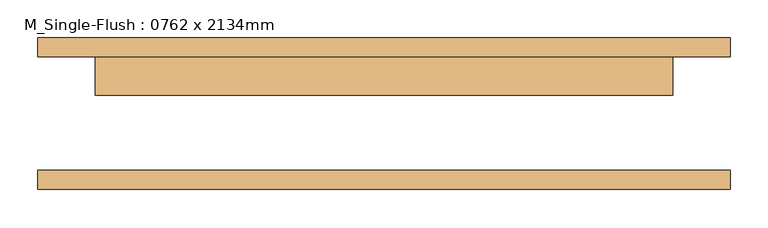
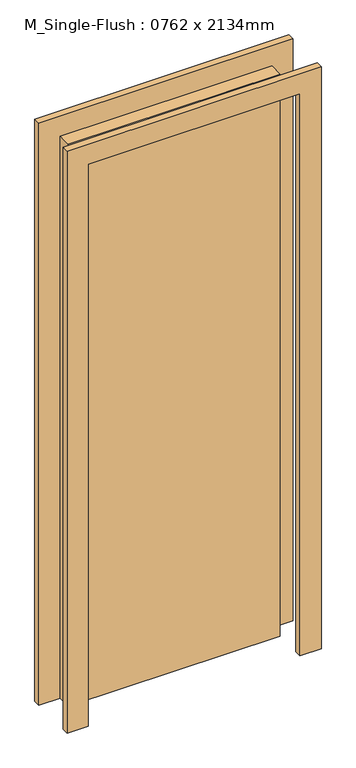
"""IFC4 building model written with IfcOpenShell, lengths in millimetres: door geometry, M_Single-Flush : 0762 x 2134mm."""

from ifc_helpers import new_model, si_unit, frame, origin, origin_with_axes, place, context, project, spatial, polyline, outline, extrude, source, transform, mapped, element, save


def m_single_flush_0762_x_2134mm_1533e4c5(model_context):
    return source(origin(), model_context, "Body", "SweptSolid", [
        extrude(outline(polyline([(2210.0, -457.0), (0.0, -457.0), (0.0, -381.0), (2134.0, -381.0), (2134.0, 381.0), (0.0, 381.0), (0.0, 457.0), (2210.0, 457.0), (2210.0, -457.0)])), frame((0.0, 75.0, 0.0), z_axis=(0.0, 1.0, 0.0), x_axis=(0.0, 0.0, 1.0)), (0.0, 0.0, 1.0), 25.0),
        extrude(outline(polyline([(2210.0, 457.0), (2210.0, -457.0), (0.0, -457.0), (0.0, -381.0), (2134.0, -381.0), (2134.0, 381.0), (0.0, 381.0), (0.0, 457.0), (2210.0, 457.0)])), frame((0.0, -100.0, 0.0), z_axis=(0.0, 1.0, 0.0), x_axis=(0.0, 0.0, 1.0)), (0.0, 0.0, 1.0), 25.0),
        extrude(outline(polyline([(381.0, 24.0), (-381.0, 24.0), (-381.0, 75.0), (381.0, 75.0), (381.0, 24.0)])), origin_with_axes(), (0.0, 0.0, 1.0), 2134.0),
    ])


if __name__ == "__main__":
    model = new_model("IFC4")
    model_context = context("Model", 3, world=origin())
    ifc_project = project(units=[si_unit("LENGTHUNIT", "METRE", prefix="MILLI")], contexts=[model_context])
    site = spatial("IfcSite", under=ifc_project)
    building = spatial("IfcBuilding", under=site)
    placement = place(None, origin())
    m_single_flush_0762_x_2134mm_shape = m_single_flush_0762_x_2134mm_1533e4c5(model_context)
    element("IfcDoor", 1, ObjectType="M_Single-Flush : 0762 x 2134mm", at=placement, inside=building, context=model_context, shape_type="MappedRepresentation", body=[
        mapped(m_single_flush_0762_x_2134mm_shape, transform((0.0, 0.0, 0.0), x_axis=(1.0, 0.0, 0.0), y_axis=(0.0, 1.0, 0.0), z_axis=(0.0, 0.0, 1.0))),
    ])
    save(model, "model.ifc")

# Revit data of these elements
# Type "M_Single-Flush : 0762 x 2134mm"
#   Type Mark = "26"
#   Construction Type Id = "MDOOR"
#   Analytic Construction = "Metal"
#   Thickness = 0.051 m
#   Thermal Resistance (R) = 0.270117 (m²·K)/W
#   Heat Transfer Coefficient (U) = 3.7021 W/(m²·K)
#   Height = 2.134 m
#   Trim Projection Ext = 0.025 m
#   Trim Projection Int = 0.025 m
#   Trim Width = 0.076 m
#   Width = 0.762 m
#   Define Thermal Properties by = 1
#   Define Thermal Properties by = 1
#   Door Material = Door - Panel
#   Frame Material = Door - Frame
#   Visual Light Transmittance = 0
#   Solar Heat Gain Coefficient = 0
#   Function = (empty or 0)
#   Wall Closure = (empty or 0)
# Element 1 (IfcDoor, "M_Single-Flush : 0762 x 2134mm")
#   Materials on its faces: "Door - Frame", "Door - Panel"
# Materials
#   "Door - Panel": class "Wood", colour RGB 210 159 95, transparency 0, Cost = 0
#   "Door - Frame": colour RGB 118 70 51, transparency 0, Cost = 0
